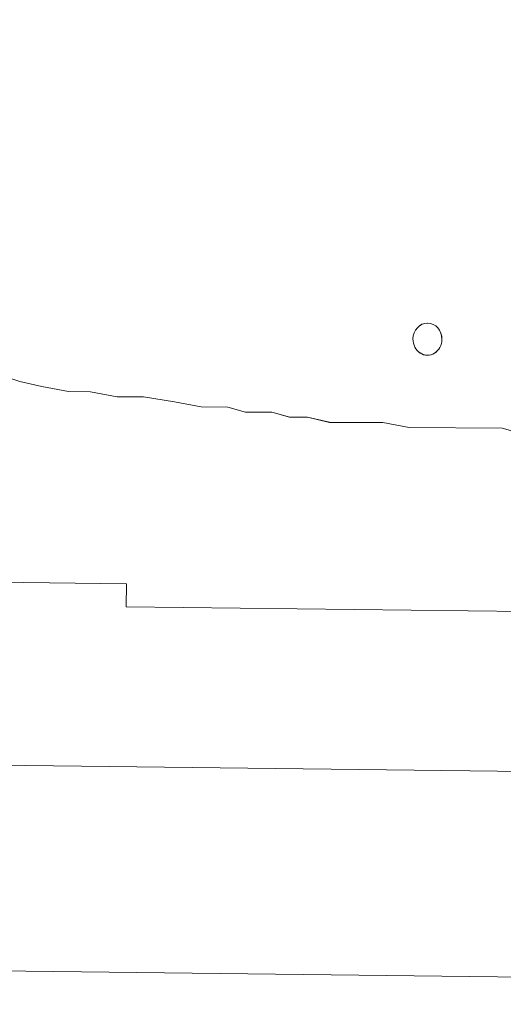
# Model space of a CAD drawing. Units: inches. Extents: x -466983 to 1020, y 324 to 318697.
# Tile 62 of 97: x 637.815 to 640.735, y 942.694 to 948.644. Entities that reach past the tile are written whole.
import ezdxf

# ---------------------------------------------------------------- set-up
doc = ezdxf.new("R2010")
doc.units = ezdxf.units.IN
doc.header["$MEASUREMENT"] = 0
doc.layers.add('A-FLOR-PATT', color=252, linetype='Continuous', lineweight=13)
doc.layers.add('A-FURN', color=8, linetype='Continuous', lineweight=18)

# ---------------------------------------------------------------- blocks, each defined once
blk = doc.blocks.new('L Shaped Sofa')
at = {"ltscale": 2}
for p, q in [((2423.757, 743.446), (2430.788, 743.36)), ((2421.46, 741.207), (2432.349, 741.074)), ((2421.666, 739.44), (2428.471, 739.357)), ((2428.471, 739.357), (2428.468, 739.105)), ((2428.468, 739.105), (2430.282, 739.083)), ((2424.133, 737.443), (2424.328, 737.388)), ((2424.328, 737.388), (2425.353, 737.383)), ((2425.353, 737.383), (2425.645, 737.327)), ((2425.645, 737.327), (2426.231, 737.325)), ((2426.231, 737.325), (2426.475, 737.269)), ((2426.475, 737.269), (2426.67, 737.268)), ((2426.67, 737.268), (2426.865, 737.213)), ((2426.865, 737.213), (2427.157, 737.212)), ((2427.157, 737.212), (2427.352, 737.157)), ((2427.352, 737.157), (2427.645, 737.155)), ((2427.645, 737.155), (2427.937, 737.1)), ((2427.937, 737.1), (2428.279, 737.044)), ((2428.279, 737.044), (2428.571, 737.043)), ((2428.571, 737.043), (2428.864, 736.987)), ((2428.864, 736.987), (2429.108, 736.986)), ((2429.108, 736.986), (2429.4, 736.93)), ((2429.4, 736.93), (2429.644, 736.875))]:
    blk.add_line(p, q, dxfattribs=at)
at = {"ltscale": 2, "extrusion": (0, 0, -1)}
for start_param, end_param in [(1.570796, 4.712389), (-1.570796, 1.570796)]:
    blk.add_ellipse((2425.152, 736.408), major_axis=(-0.002, -0.177), ratio=0.9, start_param=start_param, end_param=end_param, dxfattribs=at)

msp = doc.modelspace()

# ---------------------------------------------------------------- hatches: boundary and pattern name
at = {"layer": 'A-FLOR-PATT', "transparency": 33554572}
h = msp.add_hatch(dxfattribs=at)
h.set_pattern_fill('ANSI37', color=256, scale=30)
h.set_pattern_definition([(45, (-1212.4137, -290.035), (-2.6516504, 2.6516504), []), (135, (-1212.4137, -290.035), (-2.6516504, -2.6516504), [])])
h.paths.add_polyline_path([(901.8057, 1075.9377), (900.6144, 1075.9377), (900.6144, 1065.3856), (899.391, 1065.3856), (898.0911, 1065.3856), (892.8356, 1058.7098, -0.258377), (892.1875, 1058.3509), (879.9848, 1058.3509, -0.20177), (879.4382, 1058.5808), (874.0812, 1065.3856), (872.7813, 1065.3856), (871.5579, 1065.3856), (871.5579, 1075.9377), (813.8057, 1075.9377), (813.8057, 1044.7922), (832.3947, 1044.7922, -0.394795), (848.6602, 1028.5356), (848.6602, 1009.9377), (901.8057, 1009.9377), (901.8057, 1015.9377), (901.3057, 1015.9377), (871.3057, 1015.9377), (871.3057, 1017.2502), (871.3344, 1017.2502, -0.401453), (901.3057, 1045.9377), (901.8057, 1045.9377)])
edge = h.paths.add_edge_path(flags=16)
edge.add_line((847.7731, 1068.9486), (847.7731, 1073.7088))
edge.add_arc((849.2269, 1073.7088), 1.4538, 90, 180, ccw=False)
edge.add_line((849.2269, 1075.1627), (864.4921, 1075.1627))
edge.add_arc((864.4921, 1073.7088), 1.4538, 0, 90, ccw=False)
edge.add_line((865.9459, 1073.7088), (865.9459, 1069.0035))
edge.add_arc((832.6447, 1068.9761), 33.3012, -20.61234, 0.04725, ccw=False)
edge.add_ellipse((856.8595, 1058.48), major_axis=(0, 10.2131), ratio=0.6859192, start_angle=100.00884, end_angle=259.99116, ccw=False)
edge.add_arc((881.0742, 1068.9761), 33.3012, 180.04725, 200.61234, ccw=False)
h.paths.add_polyline_path([(853.1456, 1066.4815), (853.1456, 1066.4534), (853.1463, 1066.4534, 0.433107), (852.9166, 1066.6849), (852.9166, 1066.4534), (853.1456, 1066.4534), (853.1456, 1066.4815), (853.088, 1066.6122, 0.697939), (852.6995, 1066.4534), (852.7003, 1066.4534), (852.7003, 1066.4815), (852.9166, 1067.0012), (852.9166, 1066.6849, -0.396254)], flags=0)
h.paths.add_polyline_path([(861.0187, 1066.4815), (861.0187, 1066.4534), (861.0194, 1066.4534, 0.416404), (860.8024, 1066.6849), (860.8024, 1066.4534), (861.0187, 1066.4534), (861.0187, 1066.4815), (860.9672, 1066.6053, 0.713344), (860.5726, 1066.4534), (860.5734, 1066.4534), (860.5734, 1066.4815), (860.8024, 1067.0012), (860.8024, 1066.6849, -0.379973)], flags=0)
edge = h.paths.add_edge_path(flags=0)
edge.add_spline(control_points=[(861.1298, 1065.7855), (861.4661, 1065.2478), (861.6134, 1065.0161), (861.9833, 1064.3736), (862.1924, 1063.9443), (862.5614, 1063.0391), (862.7212, 1062.5633), (862.9865, 1061.5781), (863.092, 1061.0689), (863.2452, 1060.031), (863.293, 1059.5025), (863.3295, 1058.4409), (863.3181, 1057.9078), (863.2366, 1056.8518), (863.1664, 1056.3289), (862.9695, 1055.308), (862.8427, 1054.8099), (862.5365, 1053.8522), (862.3571, 1053.3927), (861.9514, 1052.5249), (861.7251, 1052.1166), (861.233, 1051.3622), (860.9672, 1051.0162), (860.4048, 1050.3949), (860.1082, 1050.1197), (859.4937, 1049.6461), (859.1758, 1049.4476), (858.5276, 1049.1299), (858.1973, 1049.0107), (857.5315, 1048.8518), (857.1959, 1048.8121), (856.5249, 1048.812), (856.1894, 1048.8515), (855.5236, 1049.0101), (855.1933, 1049.1291), (854.545, 1049.4465), (854.2271, 1049.6449), (853.6124, 1050.1183), (853.3158, 1050.3933), (852.7533, 1051.0143), (852.4874, 1051.3602), (851.9952, 1052.1144), (851.7688, 1052.5225), (851.3629, 1053.3902), (851.1834, 1053.8496), (850.877, 1054.8071), (850.7501, 1055.3051), (850.553, 1056.326), (850.4827, 1056.8488), (850.401, 1057.9048), (850.3895, 1058.4379), (850.4257, 1059.4995), (850.4734, 1060.0281), (850.6265, 1061.066), (850.7318, 1061.5753), (850.9969, 1062.5605), (851.1567, 1063.0365), (851.5254, 1063.9418), (851.7345, 1064.3712), (852.1056, 1065.0164), (852.2544, 1065.2503), (852.6082, 1065.7335)], knot_values=[3.915332, 3.915332, 3.915332, 3.915332, 4.013468, 4.013468, 4.175532, 4.175532, 4.337596, 4.337596, 4.49966, 4.49966, 4.661724, 4.661724, 4.823788, 4.823788, 4.985852, 4.985852, 5.147916, 5.147916, 5.30998, 5.30998, 5.472044, 5.472044, 5.634109, 5.634109, 5.796173, 5.796173, 5.958237, 5.958237, 6.120301, 6.120301, 6.282365, 6.282365, 6.444429, 6.444429, 6.606493, 6.606493, 6.768557, 6.768557, 6.930621, 6.930621, 7.092685, 7.092685, 7.254749, 7.254749, 7.416813, 7.416813, 7.578878, 7.578878, 7.740942, 7.740942, 7.903006, 7.903006, 8.06507, 8.06507, 8.227134, 8.227134, 8.389198, 8.389198, 8.551262, 8.551262, 8.65037, 8.65037, 8.65037, 8.65037], degree=3, periodic=0)
edge.add_line((852.6421, 1065.7855), (861.1298, 1065.7855))
edge = h.paths.add_edge_path(flags=0)
edge.add_ellipse((856.8496, 1057.7432), major_axis=(0, 7.7921), ratio=0.687861, start_angle=0, end_angle=360)
h.paths.add_polyline_path([(848.8634, 1069.3891), (848.8634, 1073.9605, -0.414214), (849.9538, 1075.0508), (863.7652, 1075.0508, -0.414214), (864.8555, 1073.9605), (864.8555, 1069.3891, -0.388936), (864.5237, 1069.027, -0.043561), (849.1953, 1069.027, -0.388936)], flags=0)
h.paths.add_polyline_path([(853.1006, 1068.1122, -1), (852.6775, 1068.1122, -1)], flags=0)
edge = h.paths.add_edge_path(flags=0)
edge.add_ellipse((856.8595, 1057.3378), major_axis=(0, 2.207), ratio=0.657164, start_angle=0, end_angle=360)
h.paths.add_polyline_path([(861.0415, 1068.1122, -1), (860.6184, 1068.1122, -1)], flags=0)
edge = h.paths.add_edge_path()
edge.add_line((573.9537, 1057.3412), (573.9537, 1075.9377))
edge.add_line((573.9537, 1075.9377), (558.7308, 1075.9377))
edge.add_line((558.7308, 1075.9377), (558.7308, 1065.3856))
edge.add_line((558.7308, 1065.3856), (557.5074, 1065.3856))
edge.add_line((557.5074, 1065.3856), (556.2075, 1065.3856))
edge.add_line((556.2075, 1065.3856), (550.952, 1058.7098))
edge.add_arc((550.3039, 1059.1155), 0.7646, 270, 327.94832, ccw=False)
edge.add_line((550.3039, 1058.3509), (538.1012, 1058.3509))
edge.add_arc((538.1012, 1059.1155), 0.7646, 224.3704, 270, ccw=False)
edge.add_line((537.5546, 1058.5808), (532.1976, 1065.3856))
edge.add_line((532.1976, 1065.3856), (530.8977, 1065.3856))
edge.add_line((530.8977, 1065.3856), (529.6743, 1065.3856))
edge.add_line((529.6743, 1065.3856), (529.6743, 1075.9377))
edge.add_line((529.6743, 1075.9377), (520.8057, 1075.9377))
edge.add_line((520.8057, 1075.9377), (520.8057, 1045.9377))
edge.add_line((520.8057, 1045.9377), (521.3057, 1045.9377))
edge.add_arc((521.3057, 1015.9377), 30, 2.50749, 90, ccw=False)
edge.add_line((551.277, 1017.2502), (551.3057, 1017.2502))
edge.add_line((551.3057, 1017.2502), (551.3057, 1015.9377))
edge.add_line((551.3057, 1015.9377), (520.8057, 1015.9377))
edge.add_line((520.8057, 1015.9377), (520.8057, 1009.9377))
edge.add_line((520.8057, 1009.9377), (559.1913, 1010.4022))
edge.add_arc((559.1913, 1011.856), 1.4538, 180, 270, ccw=False)
edge.add_line((557.7375, 1011.856), (557.7375, 1016.5613))
edge.add_arc((591.0386, 1016.5888), 33.3012, 159.38766, 180.04725, ccw=False)
edge.add_ellipse((566.8239, 1027.0848), major_axis=(0, 10.2131), ratio=0.6859192, start_angle=280.00884, end_angle=439.99116, ccw=False)
edge.add_arc((542.6091, 1016.5888), 33.3012, 0.04725, 20.61234, ccw=False)
edge.add_line((575.9103, 1016.6162), (575.9103, 1011.856))
edge.add_arc((574.4565, 1011.856), 1.4538, -90, 0, ccw=False)
edge.add_line((574.4565, 1010.4022), (608.8057, 1009.9377))
edge.add_line((608.8057, 1009.9377), (608.8057, 1041.0857))
edge.add_line((608.8057, 1041.0857), (590.2179, 1041.0857))
edge.add_arc((590.775, 1057.9074), 16.8309, 181.92775, 268.10321, ccw=False)
edge = h.paths.add_edge_path()
edge.add_ellipse((494.2443, 583.6204), major_axis=(0, 10.2131), ratio=0.6859192, start_angle=280.00884, end_angle=439.99116, ccw=False)
edge.add_arc((470.0296, 573.1243), 33.3012, 0.04725, 20.61234, ccw=False)
edge.add_line((503.3307, 573.1518), (503.3307, 568.3916))
edge.add_arc((501.8769, 568.3916), 1.4538, -90, 0, ccw=False)
edge.add_line((501.8769, 566.9377), (539.8057, 566.9377))
edge.add_line((539.8057, 566.9377), (539.8057, 572.9377))
edge.add_line((539.8057, 572.9377), (539.3057, 572.9377))
edge.add_line((539.3057, 572.9377), (509.3057, 572.9377))
edge.add_line((509.3057, 572.9377), (509.3057, 574.2502))
edge.add_line((509.3057, 574.2502), (509.3344, 574.2502))
edge.add_arc((539.3057, 572.9377), 30, 90, 177.49251, ccw=False)
edge.add_line((539.3057, 602.9377), (539.8057, 602.9377))
edge.add_line((539.8057, 602.9377), (539.8057, 626.9377))
edge.add_line((539.8057, 626.9377), (531.7718, 626.9377))
edge.add_line((531.7718, 626.9377), (531.7718, 616.3856))
edge.add_line((531.7718, 616.3856), (530.5484, 616.3856))
edge.add_line((530.5484, 616.3856), (529.2485, 616.3856))
edge.add_line((529.2485, 616.3856), (523.7105, 609.3509))
edge.add_line((523.7105, 609.3509), (510.7766, 609.3509))
edge.add_line((510.7766, 609.3509), (505.2386, 616.3856))
edge.add_line((505.2386, 616.3856), (503.9387, 616.3856))
edge.add_line((503.9387, 616.3856), (502.7153, 616.3856))
edge.add_line((502.7153, 616.3856), (502.7153, 626.9377))
edge.add_line((502.7153, 626.9377), (481.6983, 626.9377))
edge.add_line((481.6983, 626.9377), (481.6983, 610.995))
edge.add_arc((467.2703, 611.4728), 14.4359, 271.92775, 358.10321, ccw=False)
edge.add_line((467.7559, 597.0451), (451.8057, 597.0451))
edge.add_line((451.8057, 597.0451), (451.8057, 584.4035))
edge.add_line((451.8057, 584.4035), (451.8057, 566.9377))
edge.add_line((451.8057, 566.9377), (486.6117, 566.9377))
edge.add_arc((486.6117, 568.3916), 1.4538, 180, 270, ccw=False)
edge.add_line((485.1579, 568.3916), (485.1579, 573.0969))
edge.add_arc((518.4591, 573.1243), 33.3012, 159.38766, 180.04725, ccw=False)
h.paths.add_polyline_path([(836.2609, 1020.7328), (879.8898, 1020.7328), (879.8898, 1039.3902), (836.2609, 1039.3902)], flags=25)
h.paths.add_polyline_path([(549.9851, 1036.7492), (593.614, 1036.7492), (593.614, 1055.4065), (549.9851, 1055.4065)], flags=24)
h.paths.add_polyline_path([(475.123, 595.5959), (518.752, 595.5959), (518.752, 614.2532), (475.123, 614.2532)], flags=24)
h = msp.add_hatch(dxfattribs=at)
h.set_pattern_fill('ANSI37', color=256, scale=20)
h.set_pattern_definition([(45, (-1212.4137, -290.035), (-1.767767, 1.767767), []), (135, (-1212.4137, -290.035), (-1.767767, -1.767767), [])])
h.paths.add_polyline_path([(809.8057, 870.9377), (809.8057, 888.1519), (806.9985, 888.1519), (802.6624, 888.1519), (789.3832, 888.1519), (786.2846, 888.1519, -0.414214), (785.4991, 888.9374), (785.4991, 900.1959), (785.4991, 908.4696, -0.414214), (786.8082, 909.7787, -0.414214), (785.4991, 911.0878), (785.4991, 929.1015, -0.414214), (786.8082, 930.4106, -0.414214), (785.4991, 931.7197), (785.4991, 931.9039, -0.414214), (784.19, 930.5948), (766.7223, 930.5948, -0.412359), (765.4132, 931.8956, -0.413741), (764.1145, 930.5782), (744.5781, 930.422, -0.416556), (743.7864, 931.2075), (743.7864, 933.5153), (742.2154, 933.5153), (742.2154, 952.024, -0.001344), (743.7864, 952.1998), (743.7864, 953.9377), (678.5915, 953.9377), (678.5915, 951.1305), (678.5915, 946.7945), (678.5915, 933.5153), (678.5915, 930.4166, -0.414214), (677.806, 929.6312), (666.5475, 929.6312), (658.2738, 929.6312, -0.414214), (656.9647, 930.9403, -0.414214), (655.6556, 929.6312), (637.6419, 929.6312, -0.414214), (636.3328, 930.9403, -0.414214), (635.0237, 929.6312), (634.8395, 929.6312, -0.414214), (636.1486, 928.322), (636.1486, 910.8544, -0.412359), (634.8478, 909.5452, -0.413741), (636.1653, 908.2466), (636.3214, 888.7102, -0.416556), (635.5359, 887.9184), (633.2281, 887.9184), (633.2281, 886.3475), (614.7194, 886.3475, -0.001344), (614.5436, 887.9184), (612.8057, 887.9184), (612.8057, 834.9377), (612.8057, 752.9377), (612.8057, 748.9377), (612.8057, 697.9377), (654.8057, 697.9377), (654.8057, 701.9377), (715.8057, 701.9377), (715.8057, 737.4353), (774.2918, 737.4353), (774.2918, 795.9377), (809.8057, 795.9377)])
h.paths.add_polyline_path([(679.2761, 849.5757, 0.102523), (682.1475, 849.2608, -0.080461), (694.5428, 849.7725, -0.283899), (694.4822, 849.0082, 0.136605), (694.4068, 848.8103, -0.030441), (694.5428, 846.8929), (694.5428, 842.6198), (694.5428, 838.3466, -0.028219), (694.4246, 836.5684), (694.425, 836.5684, 0.196187), (694.4456, 836.2708, -0.302897), (694.5428, 835.467, -0.080461), (682.1475, 835.9787, 0.102523), (679.2761, 835.6638, -0.58611), (678.6457, 836.0169), (678.6457, 849.2227, -0.58611)], flags=16)
h.paths.add_polyline_path([(679.5173, 848.6515, 0.699597), (679.476, 848.6342, 1.20716), (679.1935, 848.7422, 0.010621)], flags=0)
h.paths.add_polyline_path([(679.4923, 836.5608, -0.013798), (679.9178, 836.6594, -0.071703), (682.8533, 837.1434, -0.165743), (682.1665, 839.1006), (682.1665, 842.6094), (682.1665, 846.0603, -0.240616), (683.4733, 848.6767, -0.068263), (693.9295, 849.0082), (693.7875, 848.7083), (693.7875, 849.0228, 0.067332), (683.4733, 848.6767, 0.240616), (682.1665, 846.0603), (682.1665, 842.6094), (682.1665, 839.1006, 0.23459), (683.461, 836.5513, 0.068093), (693.7875, 836.1955), (693.7875, 836.5104), (693.9296, 836.2102, -0.077215), (682.2421, 836.7815, 0.086627), (679.5283, 836.5701, -0.628402), (679.5029, 836.5735), (679.5029, 836.6071, 0.910458)], flags=0)
h.paths.add_polyline_path([(679.476, 848.6364), (679.2069, 848.647), (679.2069, 836.5718, 0.913566), (679.3645, 836.5861), (679.476, 836.5824)], flags=0)
h.paths.add_polyline_path([(679.2761, 829.8604, 0.102523), (682.1475, 829.5455, -0.080461), (694.5428, 830.0572, -0.283899), (694.4822, 829.2929, 0.136605), (694.4068, 829.095, -0.030441), (694.5428, 827.1776), (694.5428, 822.9045), (694.5428, 818.6314, -0.028219), (694.4246, 816.8531), (694.425, 816.8532, 0.196187), (694.4456, 816.5555, -0.302897), (694.5428, 815.7517, -0.080461), (682.1475, 816.2635, 0.102523), (679.2761, 815.9485, -0.58611), (678.6457, 816.3016), (678.6457, 829.5074, -0.58611)], flags=16)
h.paths.add_polyline_path([(679.5173, 828.9362, 0.699597), (679.476, 828.9189, 1.20716), (679.1935, 829.0269, 0.010621)], flags=0)
h.paths.add_polyline_path([(679.4923, 816.8456, -0.013798), (679.9178, 816.9441, -0.071703), (682.8533, 817.4281, -0.165743), (682.1665, 819.3853), (682.1665, 822.8941), (682.1665, 826.345, -0.240616), (683.4733, 828.9614, -0.068263), (693.9295, 829.2929), (693.7875, 828.9931), (693.7875, 829.3076, 0.067332), (683.4733, 828.9614, 0.240616), (682.1665, 826.345), (682.1665, 822.8941), (682.1665, 819.3853, 0.23459), (683.461, 816.836, 0.068093), (693.7875, 816.4802), (693.7875, 816.7952), (693.9296, 816.4949, -0.077215), (682.2421, 817.0662, 0.086627), (679.5283, 816.8549, -0.628402), (679.5029, 816.8582), (679.5029, 816.8918, 0.910458)], flags=0)
h.paths.add_polyline_path([(679.476, 828.9211), (679.2069, 828.9317), (679.2069, 816.8565, 0.913566), (679.3645, 816.8708), (679.476, 816.8671)], flags=0)
h.paths.add_polyline_path([(679.2761, 810.1451, 0.102523), (682.1475, 809.8302, -0.080461), (694.5428, 810.342, -0.3023), (694.4466, 809.5394, 0.10023), (694.4058, 809.3878, -0.03057), (694.5428, 807.4623), (694.5428, 803.1892), (694.5428, 798.9161, -0.03057), (694.4058, 796.9906, 0.10023), (694.4466, 796.839, -0.3023), (694.5428, 796.0365, -0.080461), (682.1475, 796.5482, 0.102523), (679.2761, 796.2333, -0.58611), (678.6457, 796.5863), (678.6457, 809.7921, -0.58611)], flags=16)
h.paths.add_polyline_path([(679.5173, 809.2417, 0.699597), (679.476, 809.2244, 1.20716), (679.1935, 809.3324, 0.010621)], flags=0)
h.paths.add_polyline_path([(679.4923, 797.151, -0.013798), (679.9178, 797.2496, -0.071703), (682.8533, 797.7336, -0.165743), (682.1665, 799.6908), (682.1665, 803.1996), (682.1665, 806.6505, -0.239349), (683.461, 809.2577, -0.072465), (694.4468, 809.5405, 0.197932), (694.425, 809.2405), (693.7875, 809.2985), (693.7875, 809.6135, 0.068093), (683.461, 809.2577, 0.239349), (682.1665, 806.6505), (682.1665, 803.1996), (682.1665, 799.6908, 0.235854), (683.4733, 797.1323, 0.067332), (693.7875, 796.7861), (693.7875, 797.1006), (694.425, 797.1586, 0.197932), (694.4468, 796.8586, -0.080419), (682.1557, 797.3795, 0.083867), (679.5283, 797.1603, -0.628402), (679.5029, 797.1637), (679.5029, 797.1973, 0.910458)], flags=0)
h.paths.add_polyline_path([(679.2069, 809.2372), (679.2069, 797.162, 0.913566), (679.3645, 797.1763), (679.476, 797.1726), (679.476, 809.2266)], flags=0)
h.paths.add_polyline_path([(695.3643, 853.2989), (728.2231, 853.2989), (728.2231, 771.1519), (695.3643, 771.1519)], flags=16)
h.paths.add_polyline_path([(696.0215, 852.6417), (727.5659, 852.6417), (727.5659, 771.809), (696.0215, 771.809)], flags=0)
h.paths.add_polyline_path([(679.2761, 788.7869, 0.102523), (682.1475, 788.472, -0.080461), (694.5428, 788.9837, -0.3023), (694.4466, 788.1812, 0.10023), (694.4058, 788.0296, -0.03057), (694.5428, 786.1041), (694.5428, 781.831), (694.5428, 777.5578, -0.03057), (694.4058, 775.6323, 0.10023), (694.4466, 775.4808, -0.3023), (694.5428, 774.6782, -0.080461), (682.1475, 775.19, 0.102523), (679.2761, 774.875, -0.58611), (678.6457, 775.2281), (678.6457, 788.4339, -0.58611)], flags=16)
h.paths.add_polyline_path([(679.5173, 787.8834, 0.699597), (679.476, 787.8662, 1.20716), (679.1935, 787.9742, 0.010621)], flags=0)
h.paths.add_polyline_path([(679.4923, 775.7928, -0.013798), (679.9178, 775.8914, -0.071703), (682.8533, 776.3753, -0.165743), (682.1665, 778.3325), (682.1665, 781.8414), (682.1665, 785.2922, -0.239349), (683.461, 787.8995, -0.072465), (694.4468, 788.1823, 0.197932), (694.425, 787.8823), (693.7875, 787.9403), (693.7875, 788.2553, 0.068093), (683.461, 787.8995, 0.239349), (682.1665, 785.2922), (682.1665, 781.8414), (682.1665, 778.3325, 0.235854), (683.4733, 775.7741, 0.067332), (693.7875, 775.4279), (693.7875, 775.7424), (694.425, 775.8004, 0.197932), (694.4468, 775.5004, -0.080419), (682.1557, 776.0212, 0.083867), (679.5283, 775.8021, -0.628402), (679.5029, 775.8054), (679.5029, 775.8391, 0.910458)], flags=0)
h.paths.add_polyline_path([(679.2069, 787.8789), (679.2069, 775.8038, 0.913566), (679.3645, 775.818), (679.476, 775.8144), (679.476, 787.8684)], flags=0)
h.paths.add_polyline_path([(704.641, 854.1204, -0.080461), (705.1527, 866.5157, 0.102523), (704.8378, 869.3871, -0.58611), (705.1908, 870.0174), (718.3966, 870.0174, -0.58611), (718.7496, 869.3871, 0.102523), (718.4347, 866.5157, -0.080461), (718.9465, 854.1204, -0.3023), (718.1439, 854.2166, 0.10023), (717.9924, 854.2574, -0.03057), (716.0668, 854.1204), (711.7937, 854.1204), (707.5206, 854.1204, -0.03057), (705.5951, 854.2574, 0.10023), (705.4435, 854.2166, -0.3023)], flags=16)
h.paths.add_polyline_path([(717.8462, 869.1459, 0.699597), (717.8289, 869.1872, 1.20716), (717.9369, 869.4697, 0.010621)], flags=0)
h.paths.add_polyline_path([(705.4631, 854.2164, -0.080419), (705.984, 866.5074, 0.083867), (705.7648, 869.1349, -0.628402), (705.7682, 869.1603), (705.8018, 869.1603, 0.910458), (705.7555, 869.1709, -0.013798), (705.8541, 868.7454, -0.071703), (706.3381, 865.8099, -0.165743), (708.2953, 866.4967), (711.8041, 866.4967), (715.255, 866.4967, -0.239349), (717.8622, 865.2022, -0.072465), (718.145, 854.2164, 0.197932), (717.845, 854.2382), (717.903, 854.8757), (718.218, 854.8757, 0.068093), (717.8622, 865.2022, 0.239349), (715.255, 866.4967), (711.8041, 866.4967), (708.2953, 866.4967, 0.235854), (705.7368, 865.1898, 0.067332), (705.3906, 854.8757), (705.7051, 854.8757), (705.7631, 854.2382, 0.197932)], flags=16)
h.paths.add_polyline_path([(705.7665, 869.4563, 0.913566), (705.7808, 869.2987), (705.7771, 869.1872), (717.8311, 869.1872), (717.8417, 869.4563)], flags=0)
h.paths.add_polyline_path([(729.0446, 842.6198), (729.0446, 846.8929, -0.03057), (729.1817, 848.8184, 0.10023), (729.1408, 848.9699, -0.3023), (729.0446, 849.7725, -0.080461), (741.4399, 849.2608, 0.102523), (744.3113, 849.5757, -0.58611), (744.9417, 849.2227), (744.9417, 836.0169, -0.58611), (744.3113, 835.6638, 0.102523), (741.4399, 835.9787, -0.080461), (729.0446, 835.467, -0.3023), (729.1408, 836.2696, 0.10023), (729.1817, 836.4211, -0.03057), (729.0446, 838.3466)], flags=16)
h.paths.add_polyline_path([(744.1115, 836.5846, 1.20716), (744.3939, 836.4766, 0.010621), (744.0701, 836.5673, 0.699597)], flags=0)
h.paths.add_polyline_path([(729.1407, 836.2684, 0.197932), (729.1624, 836.5684), (729.7999, 836.5104), (729.7999, 836.1955, 0.068093), (740.1264, 836.5513, 0.239349), (741.4209, 839.1585), (741.4209, 842.6094), (741.4209, 846.1182, 0.235854), (740.1141, 848.6767, 0.067332), (729.7999, 849.0228), (729.7999, 848.7083), (729.1624, 848.6503, 0.197932), (729.1407, 848.9504, -0.080419), (741.4317, 848.4295, 0.083867), (744.0591, 848.6486, -0.628402), (744.0845, 848.6453), (744.0845, 848.6117, 0.910458), (744.0951, 848.6579, -0.013798), (743.6696, 848.5594, -0.071703), (740.7341, 848.0754, -0.165743), (741.4209, 846.1182), (741.4209, 842.6094), (741.4209, 839.1585, -0.239349), (740.1264, 836.5513, -0.072465)], flags=0)
h.paths.add_polyline_path([(729.0446, 830.0572, -0.080461), (741.4399, 829.5455, 0.102523), (744.3113, 829.8604, -0.58611), (744.9417, 829.5074), (744.9417, 816.3016, -0.58611), (744.3113, 815.9485, 0.102523), (741.4399, 816.2635, -0.080461), (729.0446, 815.7517, -0.3023), (729.1408, 816.5543, 0.10023), (729.1817, 816.7058, -0.03057), (729.0446, 818.6314), (729.0446, 822.9045), (729.0446, 827.1776, -0.03057), (729.1817, 829.1031, 0.10023), (729.1408, 829.2547, -0.3023)], flags=16)
h.paths.add_polyline_path([(744.1115, 816.8693, 1.20716), (744.3939, 816.7613, 0.010621), (744.0701, 816.852, 0.699597)], flags=0)
h.paths.add_polyline_path([(729.1407, 829.2351, -0.080419), (741.4317, 828.7142, 0.083867), (744.0591, 828.9334, -0.628402), (744.0845, 828.93), (744.0845, 828.8964, 0.910458), (744.0951, 828.9427, -0.013798), (743.6696, 828.8441, -0.071703), (740.7341, 828.3601, -0.165743), (741.4209, 826.4029), (741.4209, 822.8941), (741.4209, 819.4432, -0.239349), (740.1264, 816.836, -0.072465), (729.1407, 816.5531, 0.197932), (729.1624, 816.8532), (729.7999, 816.7952), (729.7999, 816.4802, 0.068093), (740.1264, 816.836, 0.239349), (741.4209, 819.4432), (741.4209, 822.8941), (741.4209, 826.4029, 0.235854), (740.1141, 828.9614, 0.067332), (729.7999, 829.3076), (729.7999, 828.9931), (729.1624, 828.9351, 0.197932)], flags=16)
h.paths.add_polyline_path([(729.0446, 810.342, -0.080461), (741.4399, 809.8302, 0.102523), (744.3113, 810.1451, -0.58611), (744.9417, 809.7921), (744.9417, 796.5863, -0.58611), (744.3113, 796.2333, 0.102523), (741.4399, 796.5482, -0.080461), (729.0446, 796.0365, -0.283899), (729.1052, 796.8007, 0.136605), (729.1806, 796.9987, -0.030441), (729.0446, 798.9161), (729.0446, 803.1892), (729.0446, 807.4623, -0.028219), (729.1628, 809.2406), (729.1624, 809.2405, 0.196187), (729.1418, 809.5382, -0.302897)], flags=16)
h.paths.add_polyline_path([(744.1115, 797.1748, 1.20716), (744.3939, 797.0668, 0.010621), (744.0701, 797.1575, 0.699597)], flags=0)
h.paths.add_polyline_path([(741.3453, 809.0275, 0.086627), (744.0591, 809.2388, -0.628402), (744.0845, 809.2355), (744.0845, 809.2019, 0.910458), (744.0951, 809.2481, -0.013798), (743.6696, 809.1496, -0.071703), (740.7341, 808.6656, -0.165743), (741.4209, 806.7084), (741.4209, 803.1996), (741.4209, 799.7487, -0.240616), (740.1141, 797.1323, -0.068263), (729.658, 796.8008), (729.7999, 797.1006), (729.7999, 796.7861, 0.067332), (740.1141, 797.1323, 0.240616), (741.4209, 799.7487), (741.4209, 803.1996), (741.4209, 806.7084, 0.23459), (740.1264, 809.2577, 0.068093), (729.7999, 809.6135), (729.7999, 809.2985), (729.6578, 809.5988, -0.077215)], flags=0)
h.paths.add_polyline_path([(704.641, 770.3304, -0.283899), (705.4053, 770.2697, 0.136605), (705.6032, 770.1944, -0.030441), (707.5206, 770.3304), (711.7937, 770.3304), (716.0668, 770.3304, -0.028219), (717.8451, 770.2122), (717.845, 770.2126, 0.196187), (718.1427, 770.2331, -0.302897), (718.9465, 770.3304, -0.080461), (718.4347, 757.9351, 0.102523), (718.7496, 755.0637, -0.58611), (718.3966, 754.4333), (705.1908, 754.4333, -0.58611), (704.8378, 755.0637, 0.102523), (705.1527, 757.9351, -0.080461)], flags=16)
h.paths.add_polyline_path([(705.762, 755.3048, 0.699597), (705.7793, 755.2635, 1.20716), (705.6713, 754.9811, 0.010621)], flags=0)
h.paths.add_polyline_path([(705.4053, 769.717), (705.7051, 769.5751), (705.3906, 769.5751, 0.067332), (705.7368, 759.2609, 0.240616), (708.3532, 757.954), (711.8041, 757.954), (715.3129, 757.954, 0.23459), (717.8622, 759.2485, 0.068093), (718.218, 769.5751), (717.903, 769.5751), (718.2033, 769.7172, -0.077215), (717.632, 758.0297, 0.086627), (717.8433, 755.3159, -0.628402), (717.84, 755.2904), (717.8064, 755.2904, 0.910458), (717.8526, 755.2799, -0.013798), (717.7541, 755.7053, -0.071703), (717.2701, 758.6409, -0.165743), (715.3129, 757.954), (711.8041, 757.954), (708.3532, 757.954, -0.240616), (705.7368, 759.2609, -0.068263)], flags=0)
h.paths.add_polyline_path([(729.0446, 788.9837, -0.080461), (741.4399, 788.472, 0.102523), (744.3113, 788.7869, -0.58611), (744.9417, 788.4339), (744.9417, 775.2281, -0.58611), (744.3113, 774.875, 0.102523), (741.4399, 775.19, -0.080461), (729.0446, 774.6782, -0.283899), (729.1052, 775.4425, 0.136605), (729.1806, 775.6405, -0.030441), (729.0446, 777.5578), (729.0446, 781.831), (729.0446, 786.1041, -0.028219), (729.1628, 787.8823), (729.1624, 787.8823, 0.196187), (729.1418, 788.1799, -0.302897)], flags=16)
h.paths.add_polyline_path([(744.1115, 775.8165, 1.20716), (744.3939, 775.7086, 0.010621), (744.0701, 775.7993, 0.699597)], flags=0)
h.paths.add_polyline_path([(741.3453, 787.6692, 0.086627), (744.0591, 787.8806, -0.628402), (744.0845, 787.8773), (744.0845, 787.8437, 0.910458), (744.0951, 787.8899, -0.013798), (743.6696, 787.7913, -0.071703), (740.7341, 787.3074, -0.165743), (741.4209, 785.3502), (741.4209, 781.8414), (741.4209, 778.3905, -0.240616), (740.1141, 775.7741, -0.068263), (729.658, 775.4425), (729.7999, 775.7424), (729.7999, 775.4279, 0.067332), (740.1141, 775.7741, 0.240616), (741.4209, 778.3905), (741.4209, 781.8414), (741.4209, 785.3502, 0.23459), (740.1264, 787.8995, 0.068093), (729.7999, 788.2553), (729.7999, 787.9403), (729.6578, 788.2405, -0.077215)], flags=0)
h.paths.add_polyline_path([(744.1115, 848.6364), (744.1115, 836.5824), (744.3805, 836.5718), (744.3805, 848.647, 0.913566), (744.2229, 848.6327)], flags=0)
h.paths.add_polyline_path([(744.2229, 828.9174), (744.1115, 828.9211), (744.1115, 816.8671), (744.3805, 816.8565), (744.3805, 828.9317, 0.913566)], flags=0)
h.paths.add_polyline_path([(717.8311, 755.2635), (705.7771, 755.2635), (705.7665, 754.9945), (717.8417, 754.9945, 0.913566), (717.8274, 755.1521)], flags=0)
h.paths.add_polyline_path([(744.2229, 809.2229), (744.1115, 809.2266), (744.1115, 797.1726), (744.3805, 797.162), (744.3805, 809.2372, 0.913566)], flags=0)
h.paths.add_polyline_path([(744.1115, 787.8684), (744.1115, 775.8144), (744.3805, 775.8038), (744.3805, 787.8789, 0.913566), (744.2229, 787.8647)], flags=0)
h.paths.add_polyline_path([(678.8774, 877.1228), (737.6127, 877.1228), (737.6127, 899.5116), (678.8774, 899.5116)], flags=24)

# ---------------------------------------------------------------- linework, layer by layer
at = {"layer": 'A-FURN', "ltscale": 2}
for p, q in [((637.8147, 946.4571), (637.6278, 946.5174)), ((637.8147, 946.4571), (637.6278, 946.5174)), ((637.8147, 946.4571), (637.6278, 946.5174)), ((637.8147, 946.4571), (637.6278, 946.5174)), ((637.8147, 946.4571), (637.6278, 946.5174)), ((637.8147, 946.4571), (637.6278, 946.5174)), ((637.9482, 946.4267), (637.8147, 946.4571)), ((637.9482, 946.4267), (637.8147, 946.4571)), ((637.9482, 946.4267), (637.8147, 946.4571)), ((637.9482, 946.4267), (637.8147, 946.4571)), ((637.9482, 946.4267), (637.8147, 946.4571)), ((637.9482, 946.4267), (637.8147, 946.4571)), ((638.1086, 946.3963), (637.9482, 946.4267)), ((638.1086, 946.3963), (637.9482, 946.4267)), ((638.1086, 946.3963), (637.9482, 946.4267)), ((638.1086, 946.3963), (637.9482, 946.4267)), ((638.1086, 946.3963), (637.9482, 946.4267)), ((638.1086, 946.3963), (637.9482, 946.4267)), ((638.2423, 946.3956), (638.1086, 946.3963)), ((638.2423, 946.3956), (638.1086, 946.3963)), ((638.2423, 946.3956), (638.1086, 946.3963)), ((638.2423, 946.3956), (638.1086, 946.3963)), ((638.2423, 946.3956), (638.1086, 946.3963)), ((638.2423, 946.3956), (638.1086, 946.3963)), ((638.4026, 946.3652), (638.2423, 946.3956)), ((638.4026, 946.3652), (638.2423, 946.3956)), ((638.4026, 946.3652), (638.2423, 946.3956)), ((638.4026, 946.3652), (638.2423, 946.3956)), ((638.4026, 946.3652), (638.2423, 946.3956)), ((638.4026, 946.3652), (638.2423, 946.3956)), ((638.5631, 946.3644), (638.4026, 946.3652)), ((638.5631, 946.3644), (638.4026, 946.3652)), ((638.5631, 946.3644), (638.4026, 946.3652)), ((638.5631, 946.3644), (638.4026, 946.3652)), ((638.5631, 946.3644), (638.4026, 946.3652)), ((638.5631, 946.3644), (638.4026, 946.3652)), ((638.7502, 946.3338), (638.5631, 946.3644)), ((638.7502, 946.3338), (638.5631, 946.3644)), ((638.7502, 946.3338), (638.5631, 946.3644)), ((638.7502, 946.3338), (638.5631, 946.3644)), ((638.7502, 946.3338), (638.5631, 946.3644)), ((638.7502, 946.3338), (638.5631, 946.3644)), ((638.9105, 946.3033), (638.7502, 946.3338)), ((638.9105, 946.3033), (638.7502, 946.3338)), ((638.9105, 946.3033), (638.7502, 946.3338)), ((638.9105, 946.3033), (638.7502, 946.3338)), ((638.9105, 946.3033), (638.7502, 946.3338)), ((638.9105, 946.3033), (638.7502, 946.3338)), ((639.071, 946.3026), (638.9105, 946.3033)), ((639.071, 946.3026), (638.9105, 946.3033)), ((639.071, 946.3026), (638.9105, 946.3033)), ((639.071, 946.3026), (638.9105, 946.3033)), ((639.071, 946.3026), (638.9105, 946.3033)), ((639.071, 946.3026), (638.9105, 946.3033)), ((639.1778, 946.2724), (639.071, 946.3026)), ((639.1778, 946.2724), (639.071, 946.3026)), ((639.1778, 946.2724), (639.071, 946.3026)), ((639.1778, 946.2724), (639.071, 946.3026)), ((639.1778, 946.2724), (639.071, 946.3026)), ((639.1778, 946.2724), (639.071, 946.3026)), ((639.3383, 946.2716), (639.1778, 946.2724)), ((639.3383, 946.2716), (639.1778, 946.2724)), ((639.3383, 946.2716), (639.1778, 946.2724)), ((639.3383, 946.2716), (639.1778, 946.2724)), ((639.3383, 946.2716), (639.1778, 946.2724)), ((639.3383, 946.2716), (639.1778, 946.2724)), ((639.4452, 946.2414), (639.3383, 946.2716)), ((639.4452, 946.2414), (639.3383, 946.2716)), ((639.4452, 946.2414), (639.3383, 946.2716)), ((639.4452, 946.2414), (639.3383, 946.2716)), ((639.4452, 946.2414), (639.3383, 946.2716)), ((639.4452, 946.2414), (639.3383, 946.2716)), ((639.5522, 946.2409), (639.4452, 946.2414)), ((639.5522, 946.2409), (639.4452, 946.2414)), ((639.5522, 946.2409), (639.4452, 946.2414)), ((639.5522, 946.2409), (639.4452, 946.2414)), ((639.5522, 946.2409), (639.4452, 946.2414)), ((639.5522, 946.2409), (639.4452, 946.2414)), ((639.6857, 946.2105), (639.5522, 946.2409)), ((639.6857, 946.2105), (639.5522, 946.2409)), ((639.6857, 946.2105), (639.5522, 946.2409)), ((639.6857, 946.2105), (639.5522, 946.2409)), ((639.6857, 946.2105), (639.5522, 946.2409)), ((639.6857, 946.2105), (639.5522, 946.2409)), ((640.0067, 946.209), (639.6857, 946.2105)), ((640.0067, 946.209), (639.6857, 946.2105)), ((640.0067, 946.209), (639.6857, 946.2105)), ((640.0067, 946.209), (639.6857, 946.2105)), ((640.0067, 946.209), (639.6857, 946.2105)), ((640.0067, 946.209), (639.6857, 946.2105)), ((640.1671, 946.1785), (640.0067, 946.209)), ((640.1671, 946.1785), (640.0067, 946.209)), ((640.1671, 946.1785), (640.0067, 946.209)), ((640.1671, 946.1785), (640.0067, 946.209)), ((640.1671, 946.1785), (640.0067, 946.209)), ((640.1671, 946.1785), (640.0067, 946.209)), ((640.7288, 946.1759), (640.1671, 946.1785)), ((640.7288, 946.1759), (640.1671, 946.1785)), ((640.7288, 946.1759), (640.1671, 946.1785)), ((640.7288, 946.1759), (640.1671, 946.1785)), ((640.7288, 946.1759), (640.1671, 946.1785)), ((640.7288, 946.1759), (640.1671, 946.1785)), ((640.8356, 946.1457), (640.7288, 946.1759)), ((640.8356, 946.1457), (640.7288, 946.1759)), ((640.8356, 946.1457), (640.7288, 946.1759)), ((640.8356, 946.1457), (640.7288, 946.1759)), ((640.8356, 946.1457), (640.7288, 946.1759)), ((640.8356, 946.1457), (640.7288, 946.1759)), ((638.4594, 945.2343), (637.4646, 945.2464)), ((638.4594, 945.2343), (637.4646, 945.2464)), ((638.4594, 945.2343), (637.4646, 945.2464)), ((638.4594, 945.2343), (637.4646, 945.2464)), ((638.4594, 945.2343), (637.4646, 945.2464)), ((638.4594, 945.2343), (637.4646, 945.2464)), ((638.4577, 945.0962), (638.4594, 945.2343)), ((638.4577, 945.0962), (638.4594, 945.2343)), ((638.4577, 945.0962), (638.4594, 945.2343)), ((638.4577, 945.0962), (638.4594, 945.2343)), ((638.4577, 945.0962), (638.4594, 945.2343)), ((638.4577, 945.0962), (638.4594, 945.2343)), ((642.1884, 945.0506), (638.4577, 945.0962)), ((642.1884, 945.0506), (638.4577, 945.0962)), ((642.1884, 945.0506), (638.4577, 945.0962)), ((642.1884, 945.0506), (638.4577, 945.0962)), ((642.1884, 945.0506), (638.4577, 945.0962)), ((642.1884, 945.0506), (638.4577, 945.0962)), ((642.3009, 944.0824), (636.3319, 944.1553)), ((642.3009, 944.0824), (636.3319, 944.1553)), ((642.3009, 944.0824), (636.3319, 944.1553)), ((642.3009, 944.0824), (636.3319, 944.1553)), ((642.3009, 944.0824), (636.3319, 944.1553)), ((642.3009, 944.0824), (636.3319, 944.1553)), ((641.0422, 942.8546), (637.1872, 942.9017)), ((641.0422, 942.8546), (637.1872, 942.9017)), ((641.0422, 942.8546), (637.1872, 942.9017)), ((641.0422, 942.8546), (637.1872, 942.9017)), ((641.0422, 942.8546), (637.1872, 942.9017)), ((641.0422, 942.8546), (637.1872, 942.9017))]:
    msp.add_line(p, q, dxfattribs=at)
at = {"layer": 'A-FURN', "ltscale": 2, "extrusion": (0, 0, -1)}
for start_param, end_param in [(-1.570796, 1.570796), (-1.570796, 1.570796), (-1.570796, 1.570796), (-1.570796, 1.570796), (-1.570796, 1.570796), (-1.570796, 1.570796), (-1.570796, 1.570796), (-1.570796, 1.570796), (-1.570796, 1.570796), (-1.570796, 1.570796), (1.570796, 4.712389), (1.570796, 4.712389), (1.570796, 4.712389), (1.570796, 4.712389), (1.570796, 4.712389), (1.570796, 4.712389), (1.570796, 4.712389), (1.570796, 4.712389), (1.570796, 4.712389), (1.570796, 4.712389)]:
    msp.add_ellipse((640.2773, 946.713), major_axis=(0.0012, 0.0972), ratio=0.9, start_param=start_param, end_param=end_param, dxfattribs=at)

# ---------------------------------------------------------------- block references
at = {"layer": 'A-FURN', "xscale": 0.5482153745360612, "yscale": 0.5482153745360612, "zscale": 0.5482153745360612, "rotation": 180}
msp.add_blockref('L Shaped Sofa', (1969.7828, 1350.4232), dxfattribs=at)

doc.saveas('drawing.dxf')
